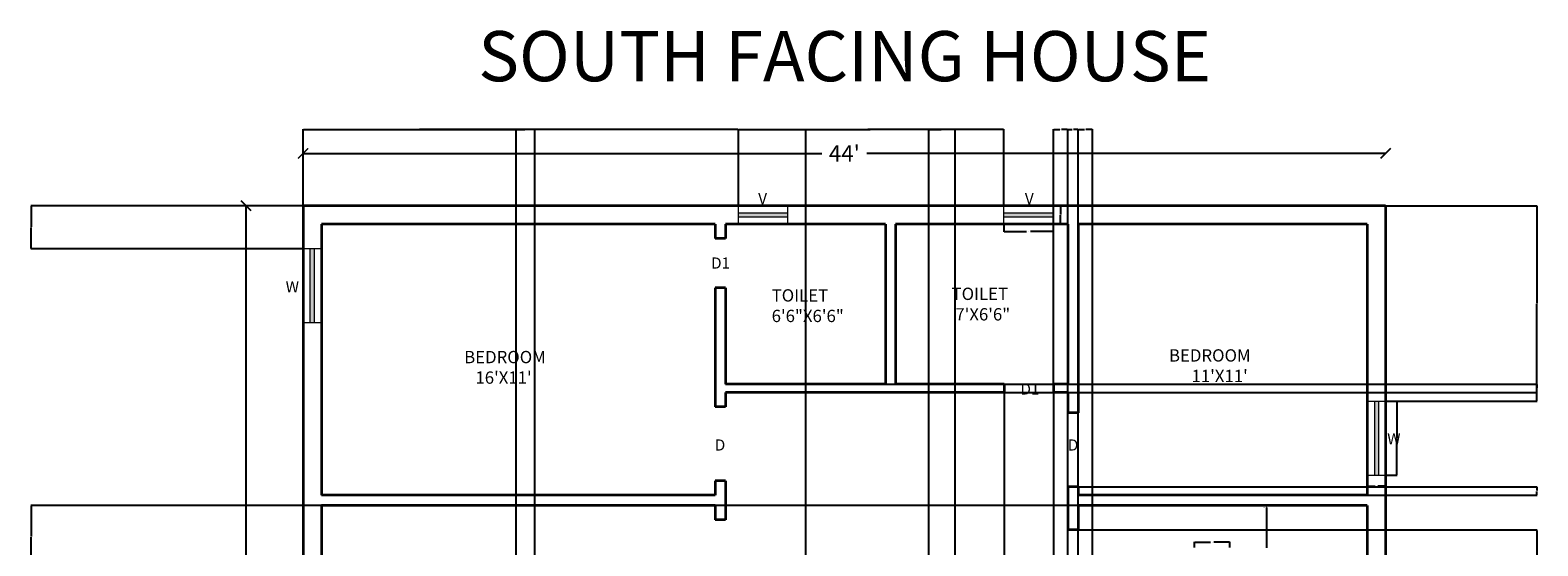
# Model space of a CAD drawing. Units: inches. Extents: x 320 to 1055, y -655 to 96.
# Tile 4 of 4: x 320 to 1055, y -155 to 96. Entities that reach past the tile are written whole.
import ezdxf

# ---------------------------------------------------------------- set-up
doc = ezdxf.new("R2010")
doc.units = ezdxf.units.IN
doc.header["$MEASUREMENT"] = 0
for name, color, linetype, lineweight in [('A-ANNO-DIMS', 2, 'Continuous', 18), ('A-ANNO-IDEN', 1, 'Continuous', 18), ('A-ANNO-TEXT', 8, 'Continuous', 18), ('A-AREA-IDEN', 8, 'Continuous', 18), ('A-GLAZ-PATT', 5, 'Continuous', 13), ('wall', 1, 'Continuous', 35), ('win', 5, 'Continuous', 18)]:
    doc.layers.add(name, color=color, linetype=linetype, lineweight=lineweight)
doc.styles.get("Standard").update_dxf_attribs({"font": 'arial.ttf'})
doc.dimstyles.get("Standard").update_dxf_attribs({"dimtxt": 0.18, "dimasz": 0.18, "dimexe": 0.18, "dimexo": 0.0625, "dimgap": 0.09, "dimtad": 0, "dimtih": 1, "dimtoh": 1, "dimdec": 1, "dimzin": 0, "dimdsep": 46, "dimlunit": 4, "dimtxsty": 'Standard', "dimcen": 0.09, "dimadec": 0, "dimazin": 0, "dimtfac": 1, "dimtdec": 1, "dimtofl": 0, "dimtmove": 0, "dimatfit": 3, "dimfxl": 1, "dimtolj": 1, "dimtzin": 0, "dimarcsym": 0})

# ---------------------------------------------------------------- blocks, each defined once
blk = doc.blocks.new('_ArchTick')
at = {"color": 0, "linetype": 'ByBlock', "const_width": 0.15}
blk.add_lwpolyline([(-0.5, -0.5), (0.5, 0.5)], dxfattribs=at)
blk = doc.blocks.new('*D1')
at = {"layer": 'A-ANNO-DIMS', "color": 0, "lineweight": -2, "transparency": 16777216}
for p, q in [((452.86, 35.74), (705.91, 35.74)), ((980.86, 35.74), (727.81, 35.74))]:
    blk.add_line(p, q, dxfattribs=at)
at = {"layer": 'Defpoints', "color": 0, "transparency": 16777216}
for p in [(980.86, 35.74), (452.86, 10.26), (980.86, 10.26)]:
    blk.add_point(p, dxfattribs=at)
at = {"layer": 'A-ANNO-DIMS', "color": 0, "lineweight": -2, "transparency": 16777216, "xscale": 5, "yscale": 5, "zscale": 5, "rotation": 180}
blk.add_blockref('_ArchTick', (452.86, 35.74), dxfattribs=at)
at = {"layer": 'A-ANNO-DIMS', "color": 0, "lineweight": -2, "transparency": 16777216, "xscale": 5, "yscale": 5, "zscale": 5}
blk.add_blockref('_ArchTick', (980.86, 35.74), dxfattribs=at)
at = {"layer": 'A-ANNO-DIMS', "color": 0, "transparency": 16777216, "insert": (716.86, 35.74), "char_height": 8, "attachment_point": 5}
blk.add_mtext("\\A1;44'", dxfattribs=at)
blk = doc.blocks.new('*D2')
at = {"layer": 'A-ANNO-DIMS', "color": 0, "lineweight": -2, "transparency": 16777216}
for p, q in [((425, 10.26), (425, -242.79)), ((425, -517.74), (425, -264.69))]:
    blk.add_line(p, q, dxfattribs=at)
at = {"layer": 'Defpoints', "color": 0, "transparency": 16777216}
for p in [(452.86, 10.26), (425, -517.74), (452.86, -517.74)]:
    blk.add_point(p, dxfattribs=at)
at = {"layer": 'A-ANNO-DIMS', "color": 0, "lineweight": -2, "transparency": 16777216, "xscale": 5, "yscale": 5, "zscale": 5}
for p, rotation in [((425, 10.26), 90), ((425, -517.74), 270)]:
    blk.add_blockref('_ArchTick', p, dxfattribs=dict(at, rotation=rotation))
at = {"layer": 'A-ANNO-DIMS', "color": 0, "transparency": 16777216, "insert": (425, -253.74), "char_height": 8, "attachment_point": 5, "rotation": 90}
blk.add_mtext("\\A1;44'", dxfattribs=at)
blk = doc.blocks.new('WINDOW-36IN')
for p, q in [((0, 36), (9, 36)), ((3.5, 36), (3.5, 0)), ((5.5, 36), (5.5, 0)), ((0, 0), (9, 0))]:
    blk.add_line(p, q)
blk = doc.blocks.new('VENT-24IN')
for p, q in [((0, 0), (0, 9)), ((24, 0), (24, 9)), ((0, 5.5), (24, 5.5)), ((0, 3.5), (24, 3.5))]:
    blk.add_line(p, q)
blk = doc.blocks.new('*D9')
at = {"layer": 'A-ANNO-DIMS', "color": 0, "lineweight": -2, "transparency": 16777216}
for p, q in [((980.92, -85.01), (986.44, -85.01)), ((986.26, -85.19), (986.26, -102.82)), ((986.26, -120.83), (986.26, -103.19)), ((980.92, -121.01), (986.44, -121.01))]:
    blk.add_line(p, q, dxfattribs=at)
at = {"layer": 'A-ANNO-DIMS', "color": 0, "transparency": 16777216}
for points in [[(986.23, -85.19), (986.29, -85.19), (986.26, -85.01)], [(986.23, -120.83), (986.29, -120.83), (986.26, -121.01)]]:
    blk.add_solid(points, dxfattribs=at)
at = {"layer": 'Defpoints', "color": 0, "transparency": 16777216}
for p in [(980.86, -85.01), (986.26, -85.01), (980.86, -121.01)]:
    blk.add_point(p, dxfattribs=at)
at = {"layer": 'A-ANNO-DIMS', "color": 0, "transparency": 16777216, "insert": (986.26, -103.01), "char_height": 0.18, "attachment_point": 5}
blk.add_mtext('\\A1;WINDOW 3\'-0" TYP.', dxfattribs=at)
blk = doc.blocks.new('*D10')
at = {"layer": 'A-ANNO-DIMS', "color": 0, "lineweight": -2, "transparency": 16777216}
for p, q in [((971.86, -121.07), (971.86, -126.59)), ((980.86, -121.07), (980.86, -126.59)), ((972.04, -126.41), (975.72, -126.41)), ((980.68, -126.41), (977, -126.41))]:
    blk.add_line(p, q, dxfattribs=at)
at = {"layer": 'A-ANNO-DIMS', "color": 0, "transparency": 16777216}
for points in [[(972.04, -126.38), (972.04, -126.44), (971.86, -126.41)], [(980.68, -126.38), (980.68, -126.44), (980.86, -126.41)]]:
    blk.add_solid(points, dxfattribs=at)
at = {"layer": 'Defpoints', "color": 0, "transparency": 16777216}
for p in [(971.86, -121.01), (980.86, -121.01), (980.86, -126.41)]:
    blk.add_point(p, dxfattribs=at)
at = {"layer": 'A-ANNO-DIMS', "color": 0, "transparency": 16777216, "insert": (976.36, -126.41), "char_height": 0.18, "attachment_point": 5}
blk.add_mtext('\\A1;0\'-9" TYP.', dxfattribs=at)
blk = doc.blocks.new('*D11')
at = {"layer": 'A-ANNO-DIMS', "color": 0, "lineweight": -2, "transparency": 16777216}
for p, q in [((794.66, 1.2), (794.66, -2.52)), ((818.66, 1.2), (818.66, -2.52)), ((794.84, -2.34), (805.64, -2.34)), ((818.48, -2.34), (807.67, -2.34))]:
    blk.add_line(p, q, dxfattribs=at)
at = {"layer": 'A-ANNO-DIMS', "color": 0, "transparency": 16777216}
for points in [[(794.84, -2.31), (794.84, -2.37), (794.66, -2.34)], [(818.48, -2.31), (818.48, -2.37), (818.66, -2.34)]]:
    blk.add_solid(points, dxfattribs=at)
at = {"layer": 'Defpoints', "color": 0, "transparency": 16777216}
for p in [(794.66, 1.26), (818.66, 1.26), (818.66, -2.34)]:
    blk.add_point(p, dxfattribs=at)
at = {"layer": 'A-ANNO-DIMS', "color": 0, "transparency": 16777216, "insert": (806.66, -2.34), "char_height": 0.18, "attachment_point": 5}
blk.add_mtext('\\A1;VENT 2\'-0" TYP.', dxfattribs=at)
blk = doc.blocks.new('*D12')
at = {"layer": 'A-ANNO-DIMS', "color": 0, "lineweight": -2, "transparency": 16777216}
for p, q in [((818.72, 10.26), (822.44, 10.26)), ((822.26, 10.08), (822.26, 5.95)), ((818.72, 1.26), (822.44, 1.26)), ((822.26, 1.44), (822.26, 5.58))]:
    blk.add_line(p, q, dxfattribs=at)
at = {"layer": 'A-ANNO-DIMS', "color": 0, "transparency": 16777216}
for points in [[(822.23, 10.08), (822.29, 10.08), (822.26, 10.26)], [(822.23, 1.44), (822.29, 1.44), (822.26, 1.26)]]:
    blk.add_solid(points, dxfattribs=at)
at = {"layer": 'Defpoints', "color": 0, "transparency": 16777216}
for p in [(818.66, 10.26), (822.26, 10.26), (818.66, 1.26)]:
    blk.add_point(p, dxfattribs=at)
at = {"layer": 'A-ANNO-DIMS', "color": 0, "transparency": 16777216, "insert": (822.26, 5.76), "char_height": 0.18, "attachment_point": 5}
blk.add_mtext('\\A1;0\'-9" TYP.', dxfattribs=at)
blk = doc.blocks.new('*D14')
at = {"layer": 'A-ANNO-DIMS', "color": 0, "lineweight": -2, "transparency": 16777216}
for p, q in [((887.57, -156.24), (887.57, -153.48)), ((887.75, -153.66), (895.4, -153.66)), ((904.73, -153.66), (897.08, -153.66)), ((904.91, -156.24), (904.91, -153.48))]:
    blk.add_line(p, q, dxfattribs=at)
at = {"layer": 'A-ANNO-DIMS', "color": 0, "transparency": 16777216}
for points in [[(887.75, -153.63), (887.75, -153.69), (887.57, -153.66)], [(904.73, -153.63), (904.73, -153.69), (904.91, -153.66)]]:
    blk.add_solid(points, dxfattribs=at)
at = {"layer": 'Defpoints', "color": 0, "transparency": 16777216}
for p in [(904.91, -153.66), (887.57, -156.31), (904.91, -156.31)]:
    blk.add_point(p, dxfattribs=at)
at = {"layer": 'A-ANNO-DIMS', "color": 0, "transparency": 16777216, "insert": (896.24, -153.66), "char_height": 0.18, "attachment_point": 5}
blk.add_mtext('\\A1;1\'-5 1/2" TYP.', dxfattribs=at)
blk = doc.blocks.new('*D21')
at = {"layer": 'A-ANNO-DIMS', "color": 0, "lineweight": -2, "transparency": 16777216}
for p, q in [((698.05, -380.67), (698.05, 47.57)), ((698.23, 47.39), (727.72, 47.39)), ((757.87, 47.39), (728.38, 47.39)), ((758.05, -380.67), (758.05, 47.57))]:
    blk.add_line(p, q, dxfattribs=at)
at = {"layer": 'A-ANNO-DIMS', "color": 0, "transparency": 16777216}
for points in [[(698.23, 47.42), (698.23, 47.36), (698.05, 47.39)], [(757.87, 47.42), (757.87, 47.36), (758.05, 47.39)]]:
    blk.add_solid(points, dxfattribs=at)
at = {"layer": 'Defpoints', "color": 0, "transparency": 16777216}
for p in [(758.05, 47.39), (698.05, -380.74), (758.05, -380.74)]:
    blk.add_point(p, dxfattribs=at)
at = {"layer": 'A-ANNO-DIMS', "color": 0, "transparency": 16777216, "insert": (728.05, 47.39), "char_height": 0.18, "attachment_point": 5}
blk.add_mtext('\\A1;5\'-0"', dxfattribs=at)
blk = doc.blocks.new('*D23')
at = {"layer": 'A-ANNO-DIMS', "color": 0, "lineweight": -2, "transparency": 16777216}
for p, q in [((794.86, -80.8), (794.86, -655.29)), ((818.86, -80.8), (818.86, -655.29)), ((795.04, -655.11), (806.53, -655.11)), ((818.68, -655.11), (807.19, -655.11))]:
    blk.add_line(p, q, dxfattribs=at)
at = {"layer": 'A-ANNO-DIMS', "color": 0, "transparency": 16777216}
for points in [[(795.04, -655.08), (795.04, -655.14), (794.86, -655.11)], [(818.68, -655.08), (818.68, -655.14), (818.86, -655.11)]]:
    blk.add_solid(points, dxfattribs=at)
at = {"layer": 'Defpoints', "color": 0, "transparency": 16777216}
for p in [(794.86, -80.74), (818.86, -80.74), (818.86, -655.11)]:
    blk.add_point(p, dxfattribs=at)
at = {"layer": 'A-ANNO-DIMS', "color": 0, "transparency": 16777216, "insert": (806.86, -655.11), "char_height": 0.18, "attachment_point": 5}
blk.add_mtext('\\A1;2\'-0"', dxfattribs=at)
blk = doc.blocks.new('*D29')
at = {"layer": 'A-ANNO-DIMS', "color": 0, "lineweight": -2, "transparency": 16777216}
for p, q in [((830.92, -147.74), (1054.75, -147.74)), ((1054.57, -147.92), (1054.57, -189.55)), ((1054.57, -231.56), (1054.57, -189.92)), ((830.92, -231.74), (1054.75, -231.74))]:
    blk.add_line(p, q, dxfattribs=at)
at = {"layer": 'A-ANNO-DIMS', "color": 0, "transparency": 16777216}
for points in [[(1054.54, -147.92), (1054.6, -147.92), (1054.57, -147.74)], [(1054.54, -231.56), (1054.6, -231.56), (1054.57, -231.74)]]:
    blk.add_solid(points, dxfattribs=at)
at = {"layer": 'Defpoints', "color": 0, "transparency": 16777216}
for p in [(830.86, -147.74), (830.86, -231.74), (1054.57, -231.74)]:
    blk.add_point(p, dxfattribs=at)
at = {"layer": 'A-ANNO-DIMS', "color": 0, "transparency": 16777216, "insert": (1054.57, -189.74), "char_height": 0.18, "attachment_point": 5}
blk.add_mtext('\\A1;7\'-0"', dxfattribs=at)
blk = doc.blocks.new('*D33')
at = {"layer": 'A-ANNO-DIMS', "color": 0, "lineweight": -2, "transparency": 16777216}
for p, q in [((452.86, -389.67), (452.86, 47.57)), ((453.04, 47.39), (509.03, 47.39)), ((565.68, 47.39), (509.69, 47.39)), ((565.86, -389.67), (565.86, 47.57))]:
    blk.add_line(p, q, dxfattribs=at)
at = {"layer": 'A-ANNO-DIMS', "color": 0, "transparency": 16777216}
for points in [[(453.04, 47.42), (453.04, 47.36), (452.86, 47.39)], [(565.68, 47.42), (565.68, 47.36), (565.86, 47.39)]]:
    blk.add_solid(points, dxfattribs=at)
at = {"layer": 'Defpoints', "color": 0, "transparency": 16777216}
for p in [(565.86, 47.39), (452.86, -389.74), (565.86, -389.74)]:
    blk.add_point(p, dxfattribs=at)
at = {"layer": 'A-ANNO-DIMS', "color": 0, "transparency": 16777216, "insert": (509.36, 47.39), "char_height": 0.18, "attachment_point": 5}
blk.add_mtext('\\A1;9\'-5"', dxfattribs=at)
blk = doc.blocks.new('*D35')
at = {"layer": 'A-ANNO-DIMS', "color": 0, "lineweight": -2, "transparency": 16777216}
for p, q in [((452.86, 10.33), (452.86, 47.57)), ((453.04, 47.39), (558.48, 47.39)), ((665.12, 47.39), (559.68, 47.39)), ((665.3, 10.33), (665.3, 47.57))]:
    blk.add_line(p, q, dxfattribs=at)
at = {"layer": 'A-ANNO-DIMS', "color": 0, "transparency": 16777216}
for points in [[(453.04, 47.42), (453.04, 47.36), (452.86, 47.39)], [(665.12, 47.42), (665.12, 47.36), (665.3, 47.39)]]:
    blk.add_solid(points, dxfattribs=at)
at = {"layer": 'Defpoints', "color": 0, "transparency": 16777216}
for p in [(665.3, 47.39), (452.86, 10.26), (665.3, 10.26)]:
    blk.add_point(p, dxfattribs=at)
at = {"layer": 'A-ANNO-DIMS', "color": 0, "transparency": 16777216, "insert": (559.08, 47.39), "char_height": 0.18, "attachment_point": 5}
blk.add_mtext('\\A1;17\'-8 1/2"', dxfattribs=at)
blk = doc.blocks.new('*D36')
at = {"layer": 'A-ANNO-DIMS', "color": 0, "lineweight": -2, "transparency": 16777216}
for p, q in [((665.3, 10.33), (665.3, 47.57)), ((665.48, 47.39), (729.38, 47.39)), ((794.48, 47.39), (730.58, 47.39)), ((794.66, 10.33), (794.66, 47.57))]:
    blk.add_line(p, q, dxfattribs=at)
at = {"layer": 'A-ANNO-DIMS', "color": 0, "transparency": 16777216}
for points in [[(665.48, 47.42), (665.48, 47.36), (665.3, 47.39)], [(794.48, 47.42), (794.48, 47.36), (794.66, 47.39)]]:
    blk.add_solid(points, dxfattribs=at)
at = {"layer": 'Defpoints', "color": 0, "transparency": 16777216}
for p in [(794.66, 47.39), (665.3, 10.26), (794.66, 10.26)]:
    blk.add_point(p, dxfattribs=at)
at = {"layer": 'A-ANNO-DIMS', "color": 0, "transparency": 16777216, "insert": (729.98, 47.39), "char_height": 0.18, "attachment_point": 5}
blk.add_mtext('\\A1;10\'-9 1/2"', dxfattribs=at)
blk = doc.blocks.new('*D37')
at = {"layer": 'A-ANNO-DIMS', "color": 0, "lineweight": -2, "transparency": 16777216}
for p, q in [((452.8, 10.26), (320.04, 10.26)), ((320.22, 10.08), (320.22, -0.08)), ((320.22, -10.61), (320.22, -0.44)), ((452.8, -10.79), (320.04, -10.79))]:
    blk.add_line(p, q, dxfattribs=at)
at = {"layer": 'A-ANNO-DIMS', "color": 0, "transparency": 16777216}
for points in [[(320.19, 10.08), (320.25, 10.08), (320.22, 10.26)], [(320.19, -10.61), (320.25, -10.61), (320.22, -10.79)]]:
    blk.add_solid(points, dxfattribs=at)
at = {"layer": 'Defpoints', "color": 0, "transparency": 16777216}
for p in [(452.86, 10.26), (320.22, -10.79), (452.86, -10.79)]:
    blk.add_point(p, dxfattribs=at)
at = {"layer": 'A-ANNO-DIMS', "color": 0, "transparency": 16777216, "insert": (320.22, -0.26), "char_height": 0.18, "attachment_point": 5}
blk.add_mtext('\\A1;1\'-9"', dxfattribs=at)
blk = doc.blocks.new('*D38')
at = {"layer": 'A-ANNO-DIMS', "color": 0, "lineweight": -2, "transparency": 16777216}
for p, q in [((980.92, 10.26), (1054.75, 10.26)), ((1054.57, 10.08), (1054.57, -37.19)), ((1054.57, -84.83), (1054.57, -37.55)), ((980.92, -85.01), (1054.75, -85.01))]:
    blk.add_line(p, q, dxfattribs=at)
at = {"layer": 'A-ANNO-DIMS', "color": 0, "transparency": 16777216}
for points in [[(1054.54, 10.08), (1054.6, 10.08), (1054.57, 10.26)], [(1054.54, -84.83), (1054.6, -84.83), (1054.57, -85.01)]]:
    blk.add_solid(points, dxfattribs=at)
at = {"layer": 'Defpoints', "color": 0, "transparency": 16777216}
for p in [(980.86, 10.26), (980.86, -85.01), (1054.57, -85.01)]:
    blk.add_point(p, dxfattribs=at)
at = {"layer": 'A-ANNO-DIMS', "color": 0, "transparency": 16777216, "insert": (1054.57, -37.37), "char_height": 0.18, "attachment_point": 5}
blk.add_mtext('\\A1;7\'-11 1/2"', dxfattribs=at)
blk = doc.blocks.new('*D40')
at = {"layer": 'A-ANNO-DIMS', "color": 0, "lineweight": -2, "transparency": 16777216}
for p, q in [((825.86, -380.67), (825.86, 47.57)), ((826.04, 47.39), (828.03, 47.39)), ((830.68, 47.39), (828.69, 47.39)), ((830.86, -380.67), (830.86, 47.57))]:
    blk.add_line(p, q, dxfattribs=at)
at = {"layer": 'A-ANNO-DIMS', "color": 0, "transparency": 16777216}
for points in [[(826.04, 47.42), (826.04, 47.36), (825.86, 47.39)], [(830.68, 47.42), (830.68, 47.36), (830.86, 47.39)]]:
    blk.add_solid(points, dxfattribs=at)
at = {"layer": 'Defpoints', "color": 0, "transparency": 16777216}
for p in [(830.86, 47.39), (825.86, -380.74), (830.86, -380.74)]:
    blk.add_point(p, dxfattribs=at)
at = {"layer": 'A-ANNO-DIMS', "color": 0, "transparency": 16777216, "insert": (828.36, 47.39), "char_height": 0.18, "attachment_point": 5}
blk.add_mtext('\\A1;0\'-5"', dxfattribs=at)
blk = doc.blocks.new('*D41')
at = {"layer": 'A-ANNO-DIMS', "color": 0, "lineweight": -2, "transparency": 16777216}
for p, q in [((971.8, -135.74), (320.04, -135.74)), ((320.22, -135.92), (320.22, -150.86)), ((320.22, -166.18), (320.22, -151.23)), ((971.8, -166.36), (320.04, -166.36))]:
    blk.add_line(p, q, dxfattribs=at)
at = {"layer": 'A-ANNO-DIMS', "color": 0, "transparency": 16777216}
for points in [[(320.19, -135.92), (320.25, -135.92), (320.22, -135.74)], [(320.19, -166.18), (320.25, -166.18), (320.22, -166.36)]]:
    blk.add_solid(points, dxfattribs=at)
at = {"layer": 'Defpoints', "color": 0, "transparency": 16777216}
for p in [(971.86, -135.74), (320.22, -166.36), (971.86, -166.36)]:
    blk.add_point(p, dxfattribs=at)
at = {"layer": 'A-ANNO-DIMS', "color": 0, "transparency": 16777216, "insert": (320.22, -151.05), "char_height": 0.18, "attachment_point": 5}
blk.add_mtext('\\A1;2\'-6 1/2"', dxfattribs=at)
blk = doc.blocks.new('*D46')
at = {"layer": 'A-ANNO-DIMS', "color": 0, "lineweight": -2, "transparency": 16777216}
for p, q in [((758.05, -380.67), (758.05, 47.57)), ((758.23, 47.39), (764.13, 47.39)), ((770.68, 47.39), (764.77, 47.39)), ((770.86, -380.67), (770.86, 47.57))]:
    blk.add_line(p, q, dxfattribs=at)
at = {"layer": 'A-ANNO-DIMS', "color": 0, "transparency": 16777216}
for points in [[(758.23, 47.42), (758.23, 47.36), (758.05, 47.39)], [(770.68, 47.42), (770.68, 47.36), (770.86, 47.39)]]:
    blk.add_solid(points, dxfattribs=at)
at = {"layer": 'Defpoints', "color": 0, "transparency": 16777216}
for p in [(770.86, 47.39), (758.05, -380.74), (770.86, -380.74)]:
    blk.add_point(p, dxfattribs=at)
at = {"layer": 'A-ANNO-DIMS', "color": 0, "transparency": 16777216, "insert": (764.45, 47.39), "char_height": 0.18, "attachment_point": 5}
blk.add_mtext('\\A1;1\'-1"', dxfattribs=at)
blk = doc.blocks.new('*D49')
at = {"layer": 'A-ANNO-DIMS', "color": 0, "lineweight": -2, "transparency": 16777216}
for p, q in [((818.86, -76.67), (818.86, 47.57)), ((819.04, 47.39), (822.03, 47.39)), ((825.68, 47.39), (822.69, 47.39)), ((825.86, -76.67), (825.86, 47.57))]:
    blk.add_line(p, q, dxfattribs=at)
at = {"layer": 'A-ANNO-DIMS', "color": 0, "transparency": 16777216}
for points in [[(819.04, 47.42), (819.04, 47.36), (818.86, 47.39)], [(825.68, 47.42), (825.68, 47.36), (825.86, 47.39)]]:
    blk.add_solid(points, dxfattribs=at)
at = {"layer": 'Defpoints', "color": 0, "transparency": 16777216}
for p in [(825.86, 47.39), (818.86, -76.74), (825.86, -76.74)]:
    blk.add_point(p, dxfattribs=at)
at = {"layer": 'A-ANNO-DIMS', "color": 0, "transparency": 16777216, "insert": (822.36, 47.39), "char_height": 0.18, "attachment_point": 5}
blk.add_mtext('\\A1;0\'-7"', dxfattribs=at)
blk = doc.blocks.new('*D50')
at = {"layer": 'A-ANNO-DIMS', "color": 0, "lineweight": -2, "transparency": 16777216}
for p, q in [((830.92, -126.74), (1054.75, -126.74)), ((830.92, -130.74), (1054.75, -130.74)), ((1054.57, -126.92), (1054.57, -128.55)), ((1054.57, -130.56), (1054.57, -128.92))]:
    blk.add_line(p, q, dxfattribs=at)
at = {"layer": 'A-ANNO-DIMS', "color": 0, "transparency": 16777216}
for points in [[(1054.54, -126.92), (1054.6, -126.92), (1054.57, -126.74)], [(1054.54, -130.56), (1054.6, -130.56), (1054.57, -130.74)]]:
    blk.add_solid(points, dxfattribs=at)
at = {"layer": 'Defpoints', "color": 0, "transparency": 16777216}
for p in [(830.86, -126.74), (830.86, -130.74), (1054.57, -126.74)]:
    blk.add_point(p, dxfattribs=at)
at = {"layer": 'A-ANNO-DIMS', "color": 0, "transparency": 16777216, "insert": (1054.57, -128.74), "char_height": 0.18, "attachment_point": 5}
blk.add_mtext('\\A1;0\'-4"', dxfattribs=at)
blk = doc.blocks.new('*D51')
at = {"layer": 'A-ANNO-DIMS', "color": 0, "lineweight": -2, "transparency": 16777216}
for p, q in [((830.86, -248.67), (830.86, 47.57)), ((831.04, 47.39), (834.03, 47.39)), ((837.68, 47.39), (834.69, 47.39)), ((837.86, -248.67), (837.86, 47.57))]:
    blk.add_line(p, q, dxfattribs=at)
at = {"layer": 'A-ANNO-DIMS', "color": 0, "transparency": 16777216}
for points in [[(831.04, 47.42), (831.04, 47.36), (830.86, 47.39)], [(837.68, 47.42), (837.68, 47.36), (837.86, 47.39)]]:
    blk.add_solid(points, dxfattribs=at)
at = {"layer": 'Defpoints', "color": 0, "transparency": 16777216}
for p in [(837.86, 47.39), (830.86, -248.74), (837.86, -248.74)]:
    blk.add_point(p, dxfattribs=at)
at = {"layer": 'A-ANNO-DIMS', "color": 0, "transparency": 16777216, "insert": (834.36, 47.39), "char_height": 0.18, "attachment_point": 5}
blk.add_mtext('\\A1;0\'-7"', dxfattribs=at)
blk = doc.blocks.new('*D52')
at = {"layer": 'A-ANNO-DIMS', "color": 0, "lineweight": -2, "transparency": 16777216}
for p, q in [((556.86, -455.67), (556.86, 47.57)), ((557.04, 47.39), (561.03, 47.39)), ((565.68, 47.39), (561.69, 47.39)), ((565.86, -423.67), (565.86, 47.57))]:
    blk.add_line(p, q, dxfattribs=at)
at = {"layer": 'A-ANNO-DIMS', "color": 0, "transparency": 16777216}
for points in [[(557.04, 47.42), (557.04, 47.36), (556.86, 47.39)], [(565.68, 47.42), (565.68, 47.36), (565.86, 47.39)]]:
    blk.add_solid(points, dxfattribs=at)
at = {"layer": 'Defpoints', "color": 0, "transparency": 16777216}
for p in [(565.86, 47.39), (565.86, -423.74), (556.86, -455.74)]:
    blk.add_point(p, dxfattribs=at)
at = {"layer": 'A-ANNO-DIMS', "color": 0, "transparency": 16777216, "insert": (561.36, 47.39), "char_height": 0.18, "attachment_point": 5}
blk.add_mtext('\\A1;0\'-9"', dxfattribs=at)
blk = doc.blocks.new('*D57')
at = {"layer": 'A-ANNO-DIMS', "color": 0, "lineweight": -2, "transparency": 16777216}
for p, q in [((658.92, -76.74), (1054.75, -76.74)), ((658.92, -80.74), (1054.75, -80.74)), ((1054.57, -76.92), (1054.57, -78.55)), ((1054.57, -80.56), (1054.57, -78.92))]:
    blk.add_line(p, q, dxfattribs=at)
at = {"layer": 'A-ANNO-DIMS', "color": 0, "transparency": 16777216}
for points in [[(1054.54, -76.92), (1054.6, -76.92), (1054.57, -76.74)], [(1054.54, -80.56), (1054.6, -80.56), (1054.57, -80.74)]]:
    blk.add_solid(points, dxfattribs=at)
at = {"layer": 'Defpoints', "color": 0, "transparency": 16777216}
for p in [(658.86, -76.74), (658.86, -80.74), (1054.57, -80.74)]:
    blk.add_point(p, dxfattribs=at)
at = {"layer": 'A-ANNO-DIMS', "color": 0, "transparency": 16777216, "insert": (1054.57, -78.74), "char_height": 0.18, "attachment_point": 5}
blk.add_mtext('\\A1;0\'-4"', dxfattribs=at)
blk = doc.blocks.new('*D59')
at = {"layer": 'A-ANNO-DIMS', "color": 0, "lineweight": -2, "transparency": 16777216}
for p, q in [((922.51, -136.87), (922.69, -136.87)), ((922.69, -136.87), (922.69, -156.46)), ((922.6, -189.59), (922.78, -189.59)), ((922.69, -189.68), (922.69, -189.5))]:
    blk.add_line(p, q, dxfattribs=at)
at = {"layer": 'A-ANNO-DIMS', "color": 0, "transparency": 16777216}
blk.add_solid([(922.72, -156.46), (922.66, -156.46), (922.69, -156.64)], dxfattribs=at)
at = {"layer": 'Defpoints', "color": 0, "transparency": 16777216}
for p in [(922.69, -156.64), (922.69, -189.59)]:
    blk.add_point(p, dxfattribs=at)
at = {"layer": 'A-ANNO-DIMS', "color": 0, "transparency": 16777216, "insert": (921.9, -136.87), "char_height": 0.18, "attachment_point": 5}
blk.add_mtext('\\A1;6X R2\'-9"', dxfattribs=at)

msp = doc.modelspace()

# ---------------------------------------------------------------- hatches: boundary and pattern name
at = {"layer": 'A-GLAZ-PATT'}
h = msp.add_hatch(color=256, dxfattribs=at)
h.dxf.hatch_style = 1
h.paths.add_polyline_path([(977.36, -166.36), (975.36, -166.36), (975.36, -214.36), (977.36, -214.36)])
h.paths.add_polyline_path([(977.36, -85.01), (975.36, -85.01), (975.36, -121.01), (977.36, -121.01)])
h.paths.add_polyline_path([(818.66, 6.76), (794.66, 6.76), (794.66, 4.76), (818.66, 4.76)])
h.paths.add_polyline_path([(689.3, 6.76), (665.3, 6.76), (665.3, 4.76), (689.3, 4.76)])
h.paths.add_polyline_path([(458.36, -10.79), (456.36, -10.79), (456.36, -46.79), (458.36, -46.79)])
h.paths.add_polyline_path([(458.36, -214.05), (456.36, -214.05), (456.36, -238.05), (458.36, -238.05)])
h.paths.add_polyline_path([(458.36, -257.01), (456.36, -257.01), (456.36, -293.01), (458.36, -293.01)])
h.paths.add_polyline_path([(977.36, -259), (975.36, -259), (975.36, -295), (977.36, -295)])
h.paths.add_polyline_path([(758.05, -384.24), (698.05, -384.24), (698.05, -386.24), (758.05, -386.24)])

# ---------------------------------------------------------------- linework, layer by layer
at = {"layer": 'wall'}
for p, q in [((452.86, 10.26), (452.86, -517.74)), ((980.86, 10.26), (452.86, 10.26)), ((452.86, 10.26), (452.86, -517.74)), ((980.86, 10.26), (980.86, -517.74)), ((461.86, 1.26), (461.86, -130.74)), ((653.86, 1.26), (461.86, 1.26)), ((653.86, 1.26), (653.86, -5.74)), ((658.86, 1.26), (658.86, -5.74)), ((736.86, 1.26), (658.86, 1.26)), ((736.86, 1.26), (736.86, -76.74)), ((741.86, 1.26), (741.86, -76.74)), ((825.86, 1.26), (741.86, 1.26)), ((825.86, 1.26), (825.86, -76.74)), ((971.86, 1.26), (830.86, 1.26)), ((830.86, 1.26), (830.86, -90.74)), ((971.86, 1.26), (971.86, -130.74)), ((658.86, -5.74), (653.86, -5.74)), ((653.86, -29.74), (653.86, -87.74)), ((658.86, -29.74), (653.86, -29.74)), ((658.86, -29.74), (658.86, -76.74)), ((736.86, -76.74), (658.86, -76.74)), ((658.86, -80.74), (658.86, -87.74)), ((794.86, -80.74), (658.86, -80.74)), ((794.86, -76.74), (741.86, -76.74)), ((794.86, -76.74), (794.86, -80.74)), ((825.86, -76.74), (818.86, -76.74)), ((818.86, -76.74), (818.86, -80.74)), ((825.86, -80.74), (818.86, -80.74)), ((825.86, -80.74), (825.86, -90.74)), ((658.86, -87.74), (653.86, -87.74)), ((830.86, -90.74), (825.86, -90.74)), ((658.86, -123.74), (653.86, -123.74)), ((653.86, -123.74), (653.86, -130.74)), ((658.86, -123.74), (658.86, -142.74)), ((653.86, -130.74), (461.86, -130.74)), ((830.86, -126.74), (825.86, -126.74)), ((825.86, -126.74), (825.86, -147.74)), ((830.86, -126.74), (830.86, -130.74)), ((971.86, -130.74), (830.86, -130.74)), ((653.86, -135.74), (461.86, -135.74)), ((461.86, -135.74), (461.86, -243.74)), ((653.86, -135.74), (653.86, -142.74)), ((971.86, -135.74), (830.86, -135.74)), ((830.86, -135.74), (830.86, -147.74)), ((971.86, -135.74), (971.86, -243.74)), ((658.86, -142.74), (653.86, -142.74)), ((830.86, -147.74), (825.86, -147.74))]:
    msp.add_line(p, q, dxfattribs=at)

# ---------------------------------------------------------------- block references
at = {"layer": 'win'}
for name, p in [('VENT-24IN', (665.3, 1.26)), ('VENT-24IN', (794.66, 1.26)), ('WINDOW-36IN', (971.86, -121.01))]:
    msp.add_blockref(name, p, dxfattribs=at)
at = {"layer": 'win', "rotation": 180}
msp.add_blockref('WINDOW-36IN', (461.86, -10.79), dxfattribs=at)

# ---------------------------------------------------------------- texts
at = {"layer": 'A-ANNO-IDEN'}
for s, height, p in [('V', 5.44, (674.85, 10.92)), ('V', 5.44, (804.93, 10.92)), ('D1', 5.444, (651.88, -20.41)), ('W', 5.44, (444.36, -31.99)), ('D1', 5.444, (802.76, -81.79)), ('W', 5.44, (981.62, -106.04)), ('D', 5.44, (653.68, -109.06)), ('D', 5.44, (825.88, -109.06))]:
    msp.add_text(s, height=height, dxfattribs=at).set_placement(p)
at = {"layer": 'A-ANNO-TEXT', "insert": (538.32, 95.33), "char_height": 24.4528, "attachment_point": 1}
msp.add_mtext_dynamic_manual_height_columns('SOUTH FACING HOUSE', width=395.3147, gutter_width=4.08, heights=[0], dxfattribs=at)
at = {"layer": 'A-AREA-IDEN', "char_height": 6, "attachment_point": 1}
for s, width, insert in [('     TOILET\\P     6\'6"X6\'6"', 54.3765, (672.24, -30.46)), ('      TOILET\\P       7\'X6\'6"', 54.3765, (758.16, -29.68)), ("   BEDROOM\\P      16'X11'", 54.3765, (525.93, -60.5)), ("BEDROOM         11'X11'", 44.9784, (875.19, -59.7))]:
    msp.add_mtext_dynamic_manual_height_columns(s, width=width, gutter_width=1, heights=[0], dxfattribs=dict(at, insert=insert))

# ---------------------------------------------------------------- dimensions: what is measured, and where the dimension line sits
at = {"layer": 'A-ANNO-DIMS'}
for base, p1, p2, picture, middle in [((665.3, 47.39), (452.86, 10.26), (665.3, 10.26), '*D35', (559.08, 47.39)), ((565.86, 47.39), (452.86, -389.74), (565.86, -389.74), '*D33', (509.36, 47.39)), ((565.86, 47.39), (556.86, -455.74), (565.86, -423.74), '*D52', (561.36, 47.39)), ((794.66, 47.39), (665.3, 10.26), (794.66, 10.26), '*D36', (729.98, 47.39)), ((758.05, 47.39), (698.05, -380.74), (758.05, -380.74), '*D21', (728.05, 47.39)), ((770.86, 47.39), (758.05, -380.74), (770.86, -380.74), '*D46', (764.45, 47.39)), ((825.86, 47.39), (818.86, -76.74), (825.86, -76.74), '*D49', (822.36, 47.39)), ((830.86, 47.39), (825.86, -380.74), (830.86, -380.74), '*D40', (828.36, 47.39)), ((837.86, 47.39), (830.86, -248.74), (837.86, -248.74), '*D51', (834.36, 47.39)), ((818.86, -655.11), (794.86, -80.74), (818.86, -80.74), '*D23', (806.86, -655.11))]:
    dim = msp.add_linear_dim(base=base, p1=p1, p2=p2, dimstyle='Standard', override={"dimdec": 1, "dimlfac": 1, "dimrnd": 0, "dimzin": 1, "dimdsep": 46, "dimlunit": 4, "dimfrac": 2}, dxfattribs=at)
    dim.commit()
    dim.dimension.update_dxf_attribs({"geometry": picture, "text_midpoint": middle})
dim = msp.add_linear_dim(base=(980.86, 35.74), p1=(452.86, 10.26), p2=(980.86, 10.26), dimstyle='Standard', override={"dimtxt": 8, "dimasz": 5, "dimgap": 4, "dimblk1": 'ArchTick', "dimblk2": 'ArchTick', "dimsah": 1, "dimse1": 1, "dimse2": 1, "dimclrd": 0, "dimclre": 0, "dimclrt": 0}, dxfattribs=at)
dim.commit()
dim.dimension.update_dxf_attribs({"geometry": '*D1', "text_midpoint": (716.86, 35.74), "dimtype": 160})
for base, p1, p2, override, picture, middle in [((320.2225, -10.7872), (452.8589, 10.2639), (452.8589, -10.7872), {"dimdec": 1, "dimlfac": 1, "dimrnd": 0, "dimzin": 1, "dimdsep": 46, "dimlunit": 4, "dimfrac": 2}, '*D37', (320.2225, -0.2617)), ((425, -517.74), (452.86, 10.26), (452.86, -517.74), {"dimtxt": 8, "dimasz": 5, "dimgap": 4, "dimtih": 0, "dimblk1": 'ArchTick', "dimblk2": 'ArchTick', "dimsah": 1, "dimse1": 1, "dimse2": 1, "dimclrd": 0, "dimclre": 0, "dimclrt": 0}, '*D2', (425, -253.74)), ((1054.57, -85.01), (980.86, 10.26), (980.86, -85.01), {"dimdec": 1, "dimlfac": 1, "dimrnd": 0, "dimzin": 1, "dimdsep": 46, "dimlunit": 4, "dimfrac": 2}, '*D38', (1054.57, -37.37)), ((1054.57, -80.74), (658.86, -76.74), (658.86, -80.74), {"dimdec": 1, "dimlfac": 1, "dimrnd": 0, "dimzin": 1, "dimdsep": 46, "dimlunit": 4, "dimfrac": 2}, '*D57', (1054.57, -78.74)), ((1054.57, -126.74), (830.86, -130.74), (830.86, -126.74), {"dimdec": 1, "dimlfac": 1, "dimrnd": 0, "dimzin": 1, "dimdsep": 46, "dimlunit": 4, "dimfrac": 2}, '*D50', (1054.57, -128.74)), ((320.22, -166.36), (971.86, -135.74), (971.86, -166.36), {"dimdec": 1, "dimlfac": 1, "dimrnd": 0, "dimzin": 1, "dimdsep": 46, "dimlunit": 4, "dimfrac": 2}, '*D41', (320.22, -151.05)), ((1054.57, -231.74), (830.86, -147.74), (830.86, -231.74), {"dimdec": 1, "dimlfac": 1, "dimrnd": 0, "dimzin": 1, "dimdsep": 46, "dimlunit": 4, "dimfrac": 2}, '*D29', (1054.57, -189.74))]:
    dim = msp.add_linear_dim(base=base, p1=p1, p2=p2, angle=90, dimstyle='Standard', override=override, dxfattribs=at)
    dim.commit()
    dim.dimension.update_dxf_attribs({"geometry": picture, "text_midpoint": middle})
for base, p1, p2, text, picture, middle in [((822.26, 10.26), (818.66, 1.26), (818.66, 10.26), '<> TYP.', '*D12', (822.26, 5.76)), ((986.26, -85.01), (980.86, -121.01), (980.86, -85.01), 'WINDOW <> TYP.', '*D9', (986.26, -103.01))]:
    dim = msp.add_linear_dim(base=base, p1=p1, p2=p2, angle=90, text=text, dimstyle='Standard', override={"dimdec": 1, "dimlfac": 1, "dimrnd": 0, "dimzin": 1, "dimdsep": 46, "dimlunit": 4, "dimfrac": 2}, dxfattribs=at)
    dim.commit()
    dim.dimension.update_dxf_attribs({"geometry": picture, "text_midpoint": middle})
for base, p1, p2, text, picture, middle in [((818.66, -2.34), (794.66, 1.26), (818.66, 1.26), 'VENT <> TYP.', '*D11', (806.66, -2.34)), ((980.86, -126.41), (971.86, -121.01), (980.86, -121.01), '<> TYP.', '*D10', (976.36, -126.41)), ((904.91, -153.66), (887.57, -156.31), (904.91, -156.31), '<> TYP.', '*D14', (896.24, -153.66))]:
    dim = msp.add_linear_dim(base=base, p1=p1, p2=p2, text=text, dimstyle='Standard', override={"dimdec": 1, "dimlfac": 1, "dimrnd": 0, "dimzin": 1, "dimdsep": 46, "dimlunit": 4, "dimfrac": 2}, dxfattribs=at)
    dim.commit()
    dim.dimension.update_dxf_attribs({"geometry": picture, "text_midpoint": middle})
dim = msp.add_radius_dim(center=(922.6941, -189.5943), mpoint=(922.694, -156.6392), text='6X <>', dimstyle='Standard', override={"dimdec": 1, "dimlfac": 1, "dimrnd": 0, "dimzin": 1, "dimdsep": 46, "dimlunit": 4, "dimfrac": 2}, dxfattribs=at)
dim.commit()
dim.dimension.update_dxf_attribs({"geometry": '*D59', "text_midpoint": (921.9047, -136.8662), "dimtype": 164})

doc.saveas('drawing.dxf')
